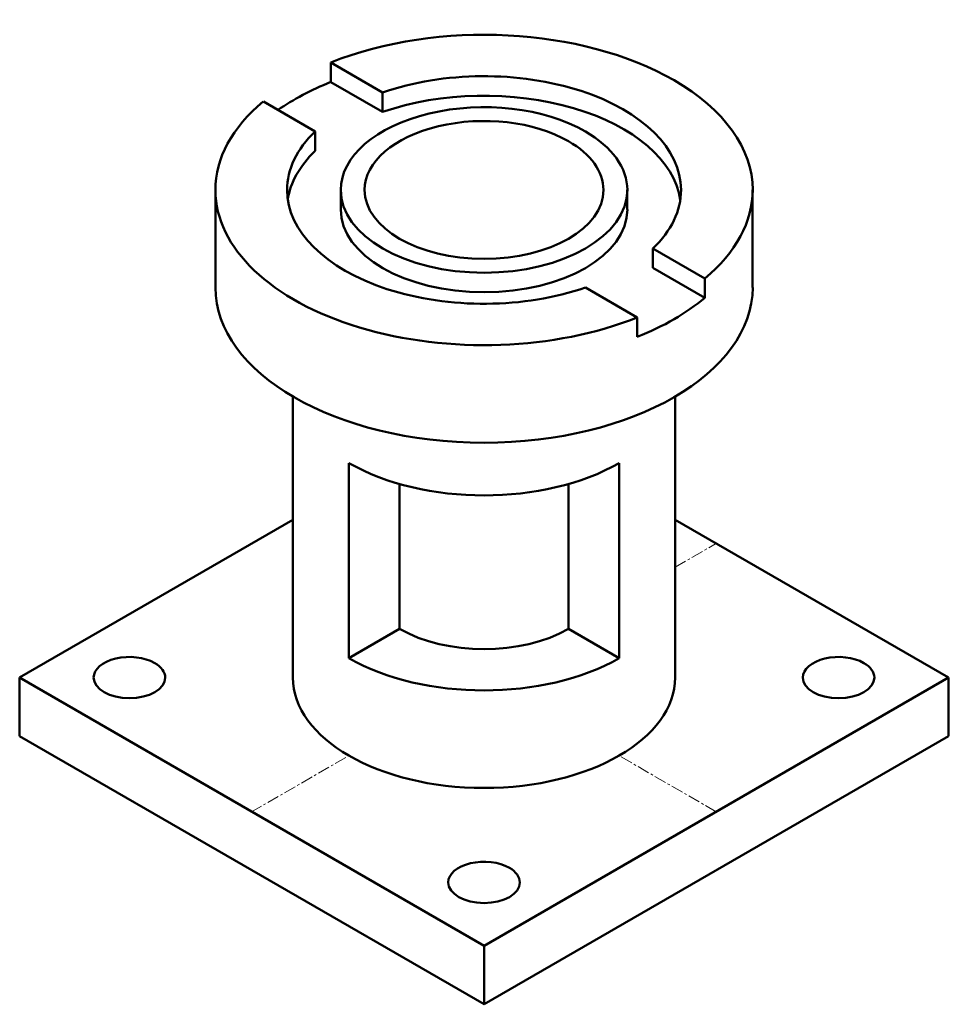
# Model space of a CAD drawing. Units: millimetres. Extents: x -1 to 95, y 29 to 130.
import ezdxf

# ---------------------------------------------------------------- set-up
doc = ezdxf.new("R2010")
doc.units = ezdxf.units.MM
doc.header["$MEASUREMENT"] = 0
doc.linetypes.add('CENTER', pattern=[2, 1.25, -0.25, 0.25, -0.25])
doc.layers.add('M-CNTR', color=4, linetype='CENTER', lineweight=18)
doc.layers.add('M-OUTL', color=7, linetype='Continuous', lineweight=50)

msp = doc.modelspace()

# ---------------------------------------------------------------- linework, layer by layer
at = {"layer": 'M-CNTR'}
for p, q in [((66.63, 74.03), (70.96, 76.52)), ((23.12, 48.9), (33.18, 54.71)), ((70.85, 48.96), (60.89, 54.71))]:
    msp.add_line(p, q, dxfattribs=at)
at = {"layer": 'M-OUTL'}
for p, q in [((31.33, 123.78), (31.33, 125.78)), ((36.64, 122.72), (31.33, 125.78)), ((36.64, 120.72), (31.33, 123.78)), ((36.64, 120.72), (36.64, 122.72)), ((29.71, 118.72), (24.4, 121.78)), ((29.71, 116.72), (29.71, 118.72)), ((19.48, 102.71), (19.48, 112.71)), ((32.34, 110.71), (32.34, 112.71)), ((61.73, 110.71), (61.73, 112.71)), ((74.59, 102.71), (74.59, 112.71)), ((69.68, 103.64), (64.36, 106.71)), ((64.36, 104.71), (64.36, 106.71)), ((69.68, 101.64), (64.36, 104.71)), ((69.68, 101.64), (69.68, 103.64)), ((62.75, 99.64), (57.44, 102.71)), ((62.75, 97.64), (62.75, 99.64)), ((27.44, 62.71), (27.44, 91.53)), ((66.63, 62.71), (66.63, 91.53)), ((33.18, 64.71), (33.18, 84.71)), ((60.89, 64.71), (60.89, 84.71)), ((38.38, 67.71), (38.38, 82.56)), ((55.7, 67.71), (55.7, 82.56)), ((-0.6, 62.71), (27.44, 78.9)), ((94.67, 62.71), (66.63, 78.9)), ((33.18, 64.71), (38.38, 67.71)), ((60.89, 64.71), (55.7, 67.71)), ((47.04, 35.21), (-0.6, 62.71)), ((-0.6, 56.71), (-0.6, 62.71)), ((47.04, 35.21), (94.67, 62.71)), ((94.67, 56.71), (94.67, 62.71)), ((47.04, 29.21), (-0.6, 56.71)), ((47.04, 29.21), (94.67, 56.71)), ((47.04, 29.21), (47.04, 35.21))]:
    msp.add_line(p, q, dxfattribs=at)
for centre, major_axis, start_param, end_param in [((47.04, 112.71), (27.56, 0), 0.785398, 2.177467), ((47.04, 112.71), (-20.21, 0), 3.141593, 5.252923), ((47.04, 110.71), (27.56, 0), 2.177467, 2.445201), ((47.04, 112.71), (27.56, 0), 0, 0.785398), ((47.04, 110.71), (20.21, 0), 0.085815, 2.111331), ((47.04, 112.71), (27.56, 0), 2.534922, 3.141593), ((47.04, 112.71), (14.7, 0), 0.785398, 3.141593), ((47.04, 112.71), (12.25, 0), 0.785398, 3.141593), ((47.04, 112.71), (-20.21, 0), 5.742651, 6.283185), ((47.04, 112.71), (14.7, 0), 0, 0.785398), ((47.04, 112.71), (12.25, 0), 0, 0.785398), ((47.04, 110.71), (20.21, 0), 2.601058, 3.055777), ((47.04, 112.71), (27.56, 0), 3.141593, 5.319059), ((47.04, 112.71), (-20.21, 0), 0, 2.111331), ((47.04, 112.71), (14.7, 0), 3.141593, 6.283185), ((47.04, 112.71), (12.25, 0), 3.141593, 6.283185), ((47.04, 112.71), (-20.21, 0), 2.601058, 3.141593), ((47.04, 112.71), (27.56, 0), 5.676515, 6.283185), ((47.04, 110.71), (14.7, 0), 3.141593, 6.283185), ((47.04, 102.71), (27.56, 0), 3.141593, 6.283185), ((47.04, 110.71), (27.56, 0), 5.319059, 5.676515), ((47.04, 92.71), (19.6, 0), 3.926991, 5.497787), ((47.04, 72.71), (12.25, 0), 3.926991, 5.497787), ((10.66, 62.71), (3.67, 0), 0.785398, 3.141593), ((47.04, 72.71), (19.6, 0), 3.926991, 5.497787), ((83.41, 62.71), (3.67, 0), 0.785398, 3.141593), ((10.66, 62.71), (3.67, 0), 0, 0.785398), ((83.41, 62.71), (3.67, 0), 0, 0.785398), ((10.66, 62.71), (3.67, 0), 3.141593, 6.283185), ((47.04, 62.71), (19.6, 0), 3.141593, 6.283185), ((83.41, 62.71), (3.67, 0), 3.141593, 6.283185), ((47.04, 41.71), (3.67, 0), 0.785398, 3.141593), ((47.04, 41.71), (3.67, 0), 0, 0.785398), ((47.04, 41.71), (3.67, 0), 3.141593, 6.283185)]:
    msp.add_ellipse(centre, major_axis=major_axis, ratio=0.57735, start_param=start_param, end_param=end_param, dxfattribs=at)

doc.saveas('drawing.dxf')
